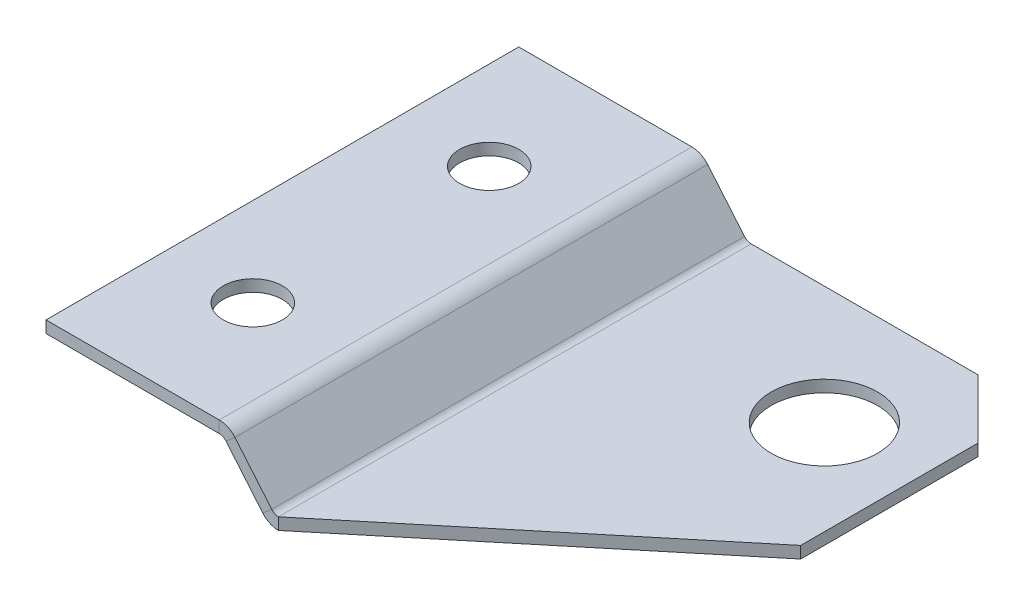
ISO-10303-21;
HEADER;
FILE_DESCRIPTION(('STEP AP214'),'2;1');
FILE_NAME('part.step','',(''),(''),'','','');
FILE_SCHEMA(('AUTOMOTIVE_DESIGN { 1 0 10303 214 1 1 1 1 }'));
ENDSEC;
DATA;
#1=APPLICATION_CONTEXT('core data for automotive mechanical design processes');
#2=APPLICATION_PROTOCOL_DEFINITION('international standard','automotive_design',2000,#1);
#3=PRODUCT_CONTEXT('',#1,'mechanical');
#4=PRODUCT('Part','Part','',(#3));
#5=PRODUCT_RELATED_PRODUCT_CATEGORY('part','',(#4));
#6=PRODUCT_DEFINITION_FORMATION('','',#4);
#7=PRODUCT_DEFINITION_CONTEXT('part definition',#1,'design');
#8=PRODUCT_DEFINITION('design','',#6,#7);
#9=PRODUCT_DEFINITION_SHAPE('','',#8);
#10=(LENGTH_UNIT() NAMED_UNIT(*) SI_UNIT(.MILLI.,.METRE.));
#11=(NAMED_UNIT(*) PLANE_ANGLE_UNIT() SI_UNIT($,.RADIAN.));
#12=(NAMED_UNIT(*) SI_UNIT($,.STERADIAN.) SOLID_ANGLE_UNIT());
#13=UNCERTAINTY_MEASURE_WITH_UNIT(LENGTH_MEASURE(1.E-05),#10,'distance_accuracy_value','');
#14=(GEOMETRIC_REPRESENTATION_CONTEXT(3) GLOBAL_UNCERTAINTY_ASSIGNED_CONTEXT((#13)) GLOBAL_UNIT_ASSIGNED_CONTEXT((#10,
#11,#12)) REPRESENTATION_CONTEXT('',''));
#15=CARTESIAN_POINT('',(0.,0.,0.));
#16=DIRECTION('',(0.,0.,1.));
#17=DIRECTION('',(1.,0.,0.));
#18=AXIS2_PLACEMENT_3D('',#15,#16,#17);
#19=CARTESIAN_POINT('',(19.3230333162743,-4.59626665871385,-40.));
#20=DIRECTION('',(0.,0.,-1.));
#21=DIRECTION('',(-1.,0.,0.));
#22=AXIS2_PLACEMENT_3D('',#19,#20,#21);
#23=PLANE('',#22);
#24=DIRECTION('',(0.642787609686543,-0.766044443118975,0.));
#25=VECTOR('',#24,1.);
#26=CARTESIAN_POINT('',(19.3230333162743,-4.59626665871385,-40.));
#27=LINE('',#26,#25);
#28=CARTESIAN_POINT('',(15.9868305589234,-0.620335037018352,-40.));
#29=VERTEX_POINT('',#28);
#30=CARTESIAN_POINT('',(19.1022472004698,-4.33314401200895,-40.));
#31=VERTEX_POINT('',#30);
#32=EDGE_CURVE('E211',#29,#31,#27,.T.);
#33=ORIENTED_EDGE('',*,*,#32,.T.);
#34=DIRECTION('',(-0.766044443118976,-0.642787609686542,0.));
#35=VECTOR('',#34,1.);
#36=CARTESIAN_POINT('',(19.1022472004698,-4.33314401200896,-40.));
#37=LINE('',#36,#35);
#38=CARTESIAN_POINT('',(18.3362027573508,-4.9759316216955,-40.));
#39=VERTEX_POINT('',#38);
#40=EDGE_CURVE('E194',#31,#39,#37,.T.);
#41=ORIENTED_EDGE('',*,*,#40,.T.);
#42=DIRECTION('',(0.642787609686543,-0.766044443118975,0.));
#43=VECTOR('',#42,1.);
#44=CARTESIAN_POINT('',(18.5569888731553,-5.23905426840039,-40.));
#45=LINE('',#44,#43);
#46=CARTESIAN_POINT('',(15.2207861158045,-1.26312264670489,-40.));
#47=VERTEX_POINT('',#46);
#48=EDGE_CURVE('E214',#47,#39,#45,.T.);
#49=ORIENTED_EDGE('',*,*,#48,.F.);
#50=DIRECTION('',(0.766044443118975,0.642787609686543,0.));
#51=VECTOR('',#50,1.);
#52=CARTESIAN_POINT('',(15.2207861158045,-1.26312264670489,-40.));
#53=LINE('',#52,#51);
#54=EDGE_CURVE('E196',#47,#29,#53,.T.);
#55=ORIENTED_EDGE('',*,*,#54,.T.);
#56=EDGE_LOOP('',(#33,#41,#49,#55));
#57=FACE_BOUND('',#56,.T.);
#58=ADVANCED_FACE('F43',(#57),#23,.T.);
#59=CARTESIAN_POINT('',(9.07600189911477,7.61566984611158,0.));
#60=DIRECTION('',(0.766044443118975,0.642787609686543,0.));
#61=DIRECTION('',(-0.642787609686543,0.766044443118975,0.));
#62=AXIS2_PLACEMENT_3D('',#59,#60,#61);
#63=PLANE('',#62);
#64=DIRECTION('',(-0.642787609686543,0.766044443118975,0.));
#65=VECTOR('',#64,1.);
#66=CARTESIAN_POINT('',(15.766044443119,-0.357212390313457,0.));
#67=LINE('',#66,#65);
#68=CARTESIAN_POINT('',(19.1022472004698,-4.33314401200896,0.));
#69=VERTEX_POINT('',#68);
#70=CARTESIAN_POINT('',(15.9868305589234,-0.620335037018351,0.));
#71=VERTEX_POINT('',#70);
#72=EDGE_CURVE('E216',#69,#71,#67,.T.);
#73=ORIENTED_EDGE('',*,*,#72,.F.);
#74=DIRECTION('',(0.,0.,-1.));
#75=VECTOR('',#74,1.);
#76=CARTESIAN_POINT('',(19.1022472004698,-4.33314401200896,-40.));
#77=LINE('',#76,#75);
#78=EDGE_CURVE('E161',#31,#69,#77,.F.);
#79=ORIENTED_EDGE('',*,*,#78,.F.);
#80=ORIENTED_EDGE('',*,*,#32,.F.);
#81=DIRECTION('',(0.,0.,1.));
#82=VECTOR('',#81,1.);
#83=CARTESIAN_POINT('',(15.9868305589234,-0.620335037018349,0.));
#84=LINE('',#83,#82);
#85=EDGE_CURVE('E206',#29,#71,#84,.T.);
#86=ORIENTED_EDGE('',*,*,#85,.T.);
#87=EDGE_LOOP('',(#73,#79,#80,#86));
#88=FACE_BOUND('',#87,.T.);
#89=ADVANCED_FACE('F301',(#88),#63,.T.);
#90=CARTESIAN_POINT('',(8.3099574559958,6.97288223642504,0.));
#91=DIRECTION('',(0.766044443118975,0.642787609686543,0.));
#92=DIRECTION('',(-0.642787609686543,0.766044443118975,0.));
#93=AXIS2_PLACEMENT_3D('',#90,#91,#92);
#94=PLANE('',#93);
#95=DIRECTION('',(0.,0.,-1.));
#96=VECTOR('',#95,1.);
#97=CARTESIAN_POINT('',(18.3362027573508,-4.9759316216955,-40.));
#98=LINE('',#97,#96);
#99=CARTESIAN_POINT('',(18.3362027573508,-4.9759316216955,0.));
#100=VERTEX_POINT('',#99);
#101=EDGE_CURVE('E188',#39,#100,#98,.F.);
#102=ORIENTED_EDGE('',*,*,#101,.T.);
#103=DIRECTION('',(-0.642787609686543,0.766044443118975,0.));
#104=VECTOR('',#103,1.);
#105=CARTESIAN_POINT('',(15.,-1.,0.));
#106=LINE('',#105,#104);
#107=CARTESIAN_POINT('',(15.2207861158045,-1.26312264670489,0.));
#108=VERTEX_POINT('',#107);
#109=EDGE_CURVE('E220',#100,#108,#106,.T.);
#110=ORIENTED_EDGE('',*,*,#109,.T.);
#111=DIRECTION('',(0.,0.,1.));
#112=VECTOR('',#111,1.);
#113=CARTESIAN_POINT('',(15.2207861158045,-1.26312264670489,-40.));
#114=LINE('',#113,#112);
#115=EDGE_CURVE('E201',#47,#108,#114,.T.);
#116=ORIENTED_EDGE('',*,*,#115,.F.);
#117=ORIENTED_EDGE('',*,*,#48,.T.);
#118=EDGE_LOOP('',(#102,#110,#116,#117));
#119=FACE_BOUND('',#118,.T.);
#120=ADVANCED_FACE('F290',(#119),#94,.F.);
#121=CARTESIAN_POINT('',(0.,-1.,0.));
#122=DIRECTION('',(0.,0.,1.));
#123=DIRECTION('',(1.,0.,0.));
#124=AXIS2_PLACEMENT_3D('',#121,#122,#123);
#125=PLANE('',#124);
#126=DIRECTION('',(1.,0.,0.));
#127=VECTOR('',#126,1.);
#128=CARTESIAN_POINT('',(0.,-1.,0.));
#129=LINE('',#128,#127);
#130=CARTESIAN_POINT('',(0.,-1.,0.));
#131=VERTEX_POINT('',#130);
#132=CARTESIAN_POINT('',(14.656517779003,-1.,0.));
#133=VERTEX_POINT('',#132);
#134=EDGE_CURVE('E248',#131,#133,#129,.T.);
#135=ORIENTED_EDGE('',*,*,#134,.T.);
#136=DIRECTION('',(0.,1.,0.));
#137=VECTOR('',#136,1.);
#138=CARTESIAN_POINT('',(14.656517779003,-1.,0.));
#139=LINE('',#138,#137);
#140=CARTESIAN_POINT('',(14.656517779003,0.,0.));
#141=VERTEX_POINT('',#140);
#142=EDGE_CURVE('E229',#133,#141,#139,.T.);
#143=ORIENTED_EDGE('',*,*,#142,.T.);
#144=DIRECTION('',(1.,0.,0.));
#145=VECTOR('',#144,1.);
#146=CARTESIAN_POINT('',(0.,0.,0.));
#147=LINE('',#146,#145);
#148=CARTESIAN_POINT('',(0.,0.,0.));
#149=VERTEX_POINT('',#148);
#150=EDGE_CURVE('E259',#149,#141,#147,.T.);
#151=ORIENTED_EDGE('',*,*,#150,.F.);
#152=DIRECTION('',(0.,1.,0.));
#153=VECTOR('',#152,1.);
#154=CARTESIAN_POINT('',(0.,-1.,0.));
#155=LINE('',#154,#153);
#156=EDGE_CURVE('E253',#131,#149,#155,.T.);
#157=ORIENTED_EDGE('',*,*,#156,.F.);
#158=EDGE_LOOP('',(#135,#143,#151,#157));
#159=FACE_BOUND('',#158,.T.);
#160=ADVANCED_FACE('F333',(#159),#125,.T.);
#161=CARTESIAN_POINT('',(0.,-1.,0.));
#162=DIRECTION('',(0.,-1.,0.));
#163=DIRECTION('',(0.,0.,-1.));
#164=AXIS2_PLACEMENT_3D('',#161,#162,#163);
#165=PLANE('',#164);
#166=CARTESIAN_POINT('',(7.5,-0.999999999999999,-10.));
#167=DIRECTION('',(0.,-1.,0.));
#168=DIRECTION('',(0.,0.,-1.));
#169=AXIS2_PLACEMENT_3D('',#166,#167,#168);
#170=CIRCLE('',#169,2.5);
#171=CARTESIAN_POINT('',(7.5,-0.999999999999999,-12.5));
#172=VERTEX_POINT('',#171);
#173=EDGE_CURVE('E158',#172,#172,#170,.T.);
#174=ORIENTED_EDGE('',*,*,#173,.F.);
#175=EDGE_LOOP('',(#174));
#176=FACE_BOUND('',#175,.T.);
#177=CARTESIAN_POINT('',(7.5,-0.999999999999999,-30.));
#178=DIRECTION('',(0.,-1.,0.));
#179=DIRECTION('',(0.,0.,-1.));
#180=AXIS2_PLACEMENT_3D('',#177,#178,#179);
#181=CIRCLE('',#180,2.5);
#182=CARTESIAN_POINT('',(7.5,-0.999999999999999,-32.5));
#183=VERTEX_POINT('',#182);
#184=EDGE_CURVE('E611',#183,#183,#181,.T.);
#185=ORIENTED_EDGE('',*,*,#184,.F.);
#186=EDGE_LOOP('',(#185));
#187=FACE_BOUND('',#186,.T.);
#188=DIRECTION('',(-1.,0.,0.));
#189=VECTOR('',#188,1.);
#190=CARTESIAN_POINT('',(0.,-1.,-40.));
#191=LINE('',#190,#189);
#192=CARTESIAN_POINT('',(14.656517779003,-1.,-40.));
#193=VERTEX_POINT('',#192);
#194=CARTESIAN_POINT('',(0.,-1.,-40.));
#195=VERTEX_POINT('',#194);
#196=EDGE_CURVE('E254',#193,#195,#191,.T.);
#197=ORIENTED_EDGE('',*,*,#196,.F.);
#198=DIRECTION('',(0.,0.,1.));
#199=VECTOR('',#198,1.);
#200=CARTESIAN_POINT('',(14.656517779003,-1.,0.));
#201=LINE('',#200,#199);
#202=EDGE_CURVE('E236',#133,#193,#201,.F.);
#203=ORIENTED_EDGE('',*,*,#202,.F.);
#204=ORIENTED_EDGE('',*,*,#134,.F.);
#205=DIRECTION('',(0.,0.,1.));
#206=VECTOR('',#205,1.);
#207=CARTESIAN_POINT('',(0.,-1.,0.));
#208=LINE('',#207,#206);
#209=EDGE_CURVE('E246',#195,#131,#208,.T.);
#210=ORIENTED_EDGE('',*,*,#209,.F.);
#211=EDGE_LOOP('',(#197,#203,#204,#210));
#212=FACE_BOUND('',#211,.T.);
#213=ADVANCED_FACE('F326',(#176,#187,#212),#165,.T.);
#214=CARTESIAN_POINT('',(0.,0.,0.));
#215=DIRECTION('',(0.,-1.,0.));
#216=DIRECTION('',(0.,0.,-1.));
#217=AXIS2_PLACEMENT_3D('',#214,#215,#216);
#218=PLANE('',#217);
#219=CARTESIAN_POINT('',(7.5,0.,-10.));
#220=DIRECTION('',(0.,1.,0.));
#221=DIRECTION('',(0.,0.,1.));
#222=AXIS2_PLACEMENT_3D('',#219,#220,#221);
#223=CIRCLE('',#222,2.5);
#224=CARTESIAN_POINT('',(7.5,0.,-7.5));
#225=VERTEX_POINT('',#224);
#226=EDGE_CURVE('E607',#225,#225,#223,.T.);
#227=ORIENTED_EDGE('',*,*,#226,.F.);
#228=EDGE_LOOP('',(#227));
#229=FACE_BOUND('',#228,.T.);
#230=CARTESIAN_POINT('',(7.5,0.,-30.));
#231=DIRECTION('',(0.,1.,0.));
#232=DIRECTION('',(0.,0.,1.));
#233=AXIS2_PLACEMENT_3D('',#230,#231,#232);
#234=CIRCLE('',#233,2.5);
#235=CARTESIAN_POINT('',(7.5,0.,-27.5));
#236=VERTEX_POINT('',#235);
#237=EDGE_CURVE('E608',#236,#236,#234,.T.);
#238=ORIENTED_EDGE('',*,*,#237,.F.);
#239=EDGE_LOOP('',(#238));
#240=FACE_BOUND('',#239,.T.);
#241=DIRECTION('',(0.,0.,1.));
#242=VECTOR('',#241,1.);
#243=CARTESIAN_POINT('',(14.656517779003,0.,0.));
#244=LINE('',#243,#242);
#245=CARTESIAN_POINT('',(14.656517779003,0.,-40.));
#246=VERTEX_POINT('',#245);
#247=EDGE_CURVE('E224',#141,#246,#244,.F.);
#248=ORIENTED_EDGE('',*,*,#247,.T.);
#249=DIRECTION('',(-1.,0.,0.));
#250=VECTOR('',#249,1.);
#251=CARTESIAN_POINT('',(0.,0.,-40.));
#252=LINE('',#251,#250);
#253=CARTESIAN_POINT('',(0.,0.,-40.));
#254=VERTEX_POINT('',#253);
#255=EDGE_CURVE('E249',#246,#254,#252,.T.);
#256=ORIENTED_EDGE('',*,*,#255,.T.);
#257=DIRECTION('',(0.,0.,1.));
#258=VECTOR('',#257,1.);
#259=CARTESIAN_POINT('',(0.,0.,0.));
#260=LINE('',#259,#258);
#261=EDGE_CURVE('E242',#254,#149,#260,.T.);
#262=ORIENTED_EDGE('',*,*,#261,.T.);
#263=ORIENTED_EDGE('',*,*,#150,.T.);
#264=EDGE_LOOP('',(#248,#256,#262,#263));
#265=FACE_BOUND('',#264,.T.);
#266=ADVANCED_FACE('F335',(#229,#240,#265),#218,.F.);
#267=CARTESIAN_POINT('',(0.,-1.,0.));
#268=DIRECTION('',(-1.,0.,0.));
#269=DIRECTION('',(0.,0.,1.));
#270=AXIS2_PLACEMENT_3D('',#267,#268,#269);
#271=PLANE('',#270);
#272=ORIENTED_EDGE('',*,*,#261,.F.);
#273=DIRECTION('',(0.,1.,0.));
#274=VECTOR('',#273,1.);
#275=CARTESIAN_POINT('',(0.,-1.,-40.));
#276=LINE('',#275,#274);
#277=EDGE_CURVE('E264',#195,#254,#276,.T.);
#278=ORIENTED_EDGE('',*,*,#277,.F.);
#279=ORIENTED_EDGE('',*,*,#209,.T.);
#280=ORIENTED_EDGE('',*,*,#156,.T.);
#281=EDGE_LOOP('',(#272,#278,#279,#280));
#282=FACE_BOUND('',#281,.T.);
#283=ADVANCED_FACE('F44',(#282),#271,.T.);
#284=CARTESIAN_POINT('',(0.,-1.,-40.));
#285=DIRECTION('',(0.,0.,-1.));
#286=DIRECTION('',(-1.,0.,0.));
#287=AXIS2_PLACEMENT_3D('',#284,#285,#286);
#288=PLANE('',#287);
#289=DIRECTION('',(0.,1.,0.));
#290=VECTOR('',#289,1.);
#291=CARTESIAN_POINT('',(14.656517779003,-1.,-40.));
#292=LINE('',#291,#290);
#293=EDGE_CURVE('E241',#193,#246,#292,.T.);
#294=ORIENTED_EDGE('',*,*,#293,.F.);
#295=ORIENTED_EDGE('',*,*,#196,.T.);
#296=ORIENTED_EDGE('',*,*,#277,.T.);
#297=ORIENTED_EDGE('',*,*,#255,.F.);
#298=EDGE_LOOP('',(#294,#295,#296,#297));
#299=FACE_BOUND('',#298,.T.);
#300=ADVANCED_FACE('F329',(#299),#288,.T.);
#301=CARTESIAN_POINT('',(14.656517779003,-1.7366,-40.));
#302=DIRECTION('',(0.,0.,-1.));
#303=DIRECTION('',(-1.,0.,0.));
#304=AXIS2_PLACEMENT_3D('',#301,#302,#303);
#305=PLANE('',#304);
#306=ORIENTED_EDGE('',*,*,#54,.F.);
#307=CARTESIAN_POINT('',(14.656517779003,-1.7366,-40.));
#308=DIRECTION('',(0.,0.,1.));
#309=DIRECTION('',(1.,0.,0.));
#310=AXIS2_PLACEMENT_3D('',#307,#308,#309);
#311=CIRCLE('',#310,0.736600000000002);
#312=EDGE_CURVE('E231',#193,#47,#311,.F.);
#313=ORIENTED_EDGE('',*,*,#312,.F.);
#314=ORIENTED_EDGE('',*,*,#293,.T.);
#315=CARTESIAN_POINT('',(14.656517779003,-1.7366,-40.));
#316=DIRECTION('',(0.,0.,1.));
#317=DIRECTION('',(1.,0.,0.));
#318=AXIS2_PLACEMENT_3D('',#315,#316,#317);
#319=CIRCLE('',#318,1.7366);
#320=EDGE_CURVE('E228',#246,#29,#319,.F.);
#321=ORIENTED_EDGE('',*,*,#320,.T.);
#322=EDGE_LOOP('',(#306,#313,#314,#321));
#323=FACE_BOUND('',#322,.T.);
#324=ADVANCED_FACE('F310',(#323),#305,.T.);
#325=CARTESIAN_POINT('',(14.656517779003,-1.7366,0.));
#326=DIRECTION('',(0.,0.,-1.));
#327=DIRECTION('',(-1.,0.,0.));
#328=AXIS2_PLACEMENT_3D('',#325,#326,#327);
#329=PLANE('',#328);
#330=CARTESIAN_POINT('',(14.656517779003,-1.7366,0.));
#331=DIRECTION('',(0.,0.,1.));
#332=DIRECTION('',(1.,0.,0.));
#333=AXIS2_PLACEMENT_3D('',#330,#331,#332);
#334=CIRCLE('',#333,0.736600000000002);
#335=EDGE_CURVE('E217',#108,#133,#334,.T.);
#336=ORIENTED_EDGE('',*,*,#335,.F.);
#337=DIRECTION('',(0.766044443118975,0.642787609686543,0.));
#338=VECTOR('',#337,1.);
#339=CARTESIAN_POINT('',(15.2207861158045,-1.26312264670489,0.));
#340=LINE('',#339,#338);
#341=EDGE_CURVE('E202',#108,#71,#340,.T.);
#342=ORIENTED_EDGE('',*,*,#341,.T.);
#343=CARTESIAN_POINT('',(14.656517779003,-1.7366,0.));
#344=DIRECTION('',(0.,0.,1.));
#345=DIRECTION('',(1.,0.,0.));
#346=AXIS2_PLACEMENT_3D('',#343,#344,#345);
#347=CIRCLE('',#346,1.7366);
#348=EDGE_CURVE('E227',#71,#141,#347,.T.);
#349=ORIENTED_EDGE('',*,*,#348,.T.);
#350=ORIENTED_EDGE('',*,*,#142,.F.);
#351=EDGE_LOOP('',(#336,#342,#349,#350));
#352=FACE_BOUND('',#351,.T.);
#353=ADVANCED_FACE('F300',(#352),#329,.F.);
#354=CARTESIAN_POINT('',(14.656517779003,-1.7366,0.));
#355=DIRECTION('',(0.,0.,1.));
#356=DIRECTION('',(0.766044443118975,0.642787609686543,0.));
#357=AXIS2_PLACEMENT_3D('',#354,#355,#356);
#358=CYLINDRICAL_SURFACE('',#357,1.7366);
#359=ORIENTED_EDGE('',*,*,#247,.F.);
#360=ORIENTED_EDGE('',*,*,#348,.F.);
#361=ORIENTED_EDGE('',*,*,#85,.F.);
#362=ORIENTED_EDGE('',*,*,#320,.F.);
#363=EDGE_LOOP('',(#359,#360,#361,#362));
#364=FACE_BOUND('',#363,.T.);
#365=ADVANCED_FACE('F304',(#364),#358,.T.);
#366=CARTESIAN_POINT('',(14.656517779003,-1.7366,0.));
#367=DIRECTION('',(0.,0.,1.));
#368=DIRECTION('',(0.766044443118975,0.642787609686543,0.));
#369=AXIS2_PLACEMENT_3D('',#366,#367,#368);
#370=CYLINDRICAL_SURFACE('',#369,0.736600000000002);
#371=ORIENTED_EDGE('',*,*,#202,.T.);
#372=ORIENTED_EDGE('',*,*,#312,.T.);
#373=ORIENTED_EDGE('',*,*,#115,.T.);
#374=ORIENTED_EDGE('',*,*,#335,.T.);
#375=EDGE_LOOP('',(#371,#372,#373,#374));
#376=FACE_BOUND('',#375,.T.);
#377=ADVANCED_FACE('F325',(#376),#370,.F.);
#378=CARTESIAN_POINT('',(15.766044443119,-0.357212390313457,0.));
#379=DIRECTION('',(0.,0.,1.));
#380=DIRECTION('',(1.,0.,0.));
#381=AXIS2_PLACEMENT_3D('',#378,#379,#380);
#382=PLANE('',#381);
#383=DIRECTION('',(-0.766044443118976,-0.642787609686542,0.));
#384=VECTOR('',#383,1.);
#385=CARTESIAN_POINT('',(19.1022472004698,-4.33314401200896,0.));
#386=LINE('',#385,#384);
#387=EDGE_CURVE('E197',#69,#100,#386,.T.);
#388=ORIENTED_EDGE('',*,*,#387,.F.);
#389=ORIENTED_EDGE('',*,*,#72,.T.);
#390=ORIENTED_EDGE('',*,*,#341,.F.);
#391=ORIENTED_EDGE('',*,*,#109,.F.);
#392=EDGE_LOOP('',(#388,#389,#390,#391));
#393=FACE_BOUND('',#392,.T.);
#394=ADVANCED_FACE('F292',(#393),#382,.T.);
#395=CARTESIAN_POINT('',(19.6665155372712,-3.85966665871385,0.));
#396=DIRECTION('',(0.,0.,1.));
#397=DIRECTION('',(1.,0.,0.));
#398=AXIS2_PLACEMENT_3D('',#395,#396,#397);
#399=PLANE('',#398);
#400=DIRECTION('',(0.,-1.,0.));
#401=VECTOR('',#400,1.);
#402=CARTESIAN_POINT('',(19.6665155372712,-4.59626665871385,0.));
#403=LINE('',#402,#401);
#404=CARTESIAN_POINT('',(19.6665155372712,-4.59626665871385,0.));
#405=VERTEX_POINT('',#404);
#406=CARTESIAN_POINT('',(19.6665155372712,-5.59626665871385,0.));
#407=VERTEX_POINT('',#406);
#408=EDGE_CURVE('E140',#405,#407,#403,.T.);
#409=ORIENTED_EDGE('',*,*,#408,.F.);
#410=CARTESIAN_POINT('',(19.6665155372712,-3.85966665871385,0.));
#411=DIRECTION('',(0.,0.,-1.));
#412=DIRECTION('',(-1.,0.,0.));
#413=AXIS2_PLACEMENT_3D('',#410,#411,#412);
#414=CIRCLE('',#413,0.736599999999999);
#415=EDGE_CURVE('E151',#69,#405,#414,.F.);
#416=ORIENTED_EDGE('',*,*,#415,.F.);
#417=ORIENTED_EDGE('',*,*,#387,.T.);
#418=CARTESIAN_POINT('',(19.6665155372712,-3.85966665871385,0.));
#419=DIRECTION('',(0.,0.,-1.));
#420=DIRECTION('',(-1.,0.,0.));
#421=AXIS2_PLACEMENT_3D('',#418,#419,#420);
#422=CIRCLE('',#421,1.7366);
#423=EDGE_CURVE('E153',#100,#407,#422,.F.);
#424=ORIENTED_EDGE('',*,*,#423,.T.);
#425=EDGE_LOOP('',(#409,#416,#417,#424));
#426=FACE_BOUND('',#425,.T.);
#427=ADVANCED_FACE('F148',(#426),#399,.T.);
#428=CARTESIAN_POINT('',(19.6665155372712,-3.85966665871385,-40.));
#429=DIRECTION('',(0.,0.,1.));
#430=DIRECTION('',(1.,0.,0.));
#431=AXIS2_PLACEMENT_3D('',#428,#429,#430);
#432=PLANE('',#431);
#433=CARTESIAN_POINT('',(19.6665155372712,-3.85966665871385,-40.));
#434=DIRECTION('',(0.,0.,-1.));
#435=DIRECTION('',(-1.,0.,0.));
#436=AXIS2_PLACEMENT_3D('',#433,#434,#435);
#437=CIRCLE('',#436,0.736599999999999);
#438=CARTESIAN_POINT('',(19.6665155372712,-4.59626665871385,-40.));
#439=VERTEX_POINT('',#438);
#440=EDGE_CURVE('E190',#439,#31,#437,.T.);
#441=ORIENTED_EDGE('',*,*,#440,.F.);
#442=DIRECTION('',(0.,-1.,0.));
#443=VECTOR('',#442,1.);
#444=CARTESIAN_POINT('',(19.6665155372712,-4.59626665871385,-40.));
#445=LINE('',#444,#443);
#446=CARTESIAN_POINT('',(19.6665155372712,-5.59626665871385,-40.));
#447=VERTEX_POINT('',#446);
#448=EDGE_CURVE('E167',#439,#447,#445,.T.);
#449=ORIENTED_EDGE('',*,*,#448,.T.);
#450=CARTESIAN_POINT('',(19.6665155372712,-3.85966665871385,-40.));
#451=DIRECTION('',(0.,0.,-1.));
#452=DIRECTION('',(-1.,0.,0.));
#453=AXIS2_PLACEMENT_3D('',#450,#451,#452);
#454=CIRCLE('',#453,1.7366);
#455=EDGE_CURVE('E165',#447,#39,#454,.T.);
#456=ORIENTED_EDGE('',*,*,#455,.T.);
#457=ORIENTED_EDGE('',*,*,#40,.F.);
#458=EDGE_LOOP('',(#441,#449,#456,#457));
#459=FACE_BOUND('',#458,.T.);
#460=ADVANCED_FACE('F279',(#459),#432,.F.);
#461=CARTESIAN_POINT('',(19.6665155372712,-3.85966665871385,-40.));
#462=DIRECTION('',(0.,0.,-1.));
#463=DIRECTION('',(0.,-1.,0.));
#464=AXIS2_PLACEMENT_3D('',#461,#462,#463);
#465=CYLINDRICAL_SURFACE('',#464,1.7366);
#466=ORIENTED_EDGE('',*,*,#101,.F.);
#467=ORIENTED_EDGE('',*,*,#455,.F.);
#468=DIRECTION('',(0.,0.,1.));
#469=VECTOR('',#468,1.);
#470=CARTESIAN_POINT('',(19.6665155372712,-5.59626665871385,0.));
#471=LINE('',#470,#469);
#472=EDGE_CURVE('E173',#447,#407,#471,.T.);
#473=ORIENTED_EDGE('',*,*,#472,.T.);
#474=ORIENTED_EDGE('',*,*,#423,.F.);
#475=EDGE_LOOP('',(#466,#467,#473,#474));
#476=FACE_BOUND('',#475,.T.);
#477=ADVANCED_FACE('F283',(#476),#465,.T.);
#478=CARTESIAN_POINT('',(19.6665155372712,-3.85966665871385,-40.));
#479=DIRECTION('',(0.,0.,-1.));
#480=DIRECTION('',(0.,-1.,0.));
#481=AXIS2_PLACEMENT_3D('',#478,#479,#480);
#482=CYLINDRICAL_SURFACE('',#481,0.736599999999999);
#483=ORIENTED_EDGE('',*,*,#78,.T.);
#484=ORIENTED_EDGE('',*,*,#415,.T.);
#485=DIRECTION('',(0.,0.,-1.));
#486=VECTOR('',#485,1.);
#487=CARTESIAN_POINT('',(19.6665155372712,-4.59626665871385,0.));
#488=LINE('',#487,#486);
#489=EDGE_CURVE('E152',#405,#439,#488,.T.);
#490=ORIENTED_EDGE('',*,*,#489,.T.);
#491=ORIENTED_EDGE('',*,*,#440,.T.);
#492=EDGE_LOOP('',(#483,#484,#490,#491));
#493=FACE_BOUND('',#492,.T.);
#494=ADVANCED_FACE('F157',(#493),#482,.F.);
#495=CARTESIAN_POINT('',(43.8567256581193,-5.59626665871385,-40.));
#496=DIRECTION('',(0.,0.,1.));
#497=DIRECTION('',(1.,0.,0.));
#498=AXIS2_PLACEMENT_3D('',#495,#496,#497);
#499=PLANE('',#498);
#500=DIRECTION('',(1.,0.,0.));
#501=VECTOR('',#500,1.);
#502=CARTESIAN_POINT('',(43.8567256581193,-4.59626665871385,-40.));
#503=LINE('',#502,#501);
#504=CARTESIAN_POINT('',(38.8567256581193,-4.59626665871385,-40.));
#505=VERTEX_POINT('',#504);
#506=EDGE_CURVE('E169',#439,#505,#503,.T.);
#507=ORIENTED_EDGE('',*,*,#506,.T.);
#508=DIRECTION('',(0.,1.,0.));
#509=VECTOR('',#508,1.);
#510=CARTESIAN_POINT('',(38.8567256581193,-14.5962666587139,-40.));
#511=LINE('',#510,#509);
#512=CARTESIAN_POINT('',(38.8567256581193,-5.59626665871385,-40.));
#513=VERTEX_POINT('',#512);
#514=EDGE_CURVE('E144',#513,#505,#511,.T.);
#515=ORIENTED_EDGE('',*,*,#514,.F.);
#516=DIRECTION('',(1.,0.,0.));
#517=VECTOR('',#516,1.);
#518=CARTESIAN_POINT('',(43.8567256581193,-5.59626665871385,-40.));
#519=LINE('',#518,#517);
#520=EDGE_CURVE('E179',#447,#513,#519,.T.);
#521=ORIENTED_EDGE('',*,*,#520,.F.);
#522=ORIENTED_EDGE('',*,*,#448,.F.);
#523=EDGE_LOOP('',(#507,#515,#521,#522));
#524=FACE_BOUND('',#523,.T.);
#525=ADVANCED_FACE('F274',(#524),#499,.F.);
#526=CARTESIAN_POINT('',(0.,-5.59626665871384,0.));
#527=DIRECTION('',(0.,1.,0.));
#528=DIRECTION('',(-1.,0.,0.));
#529=AXIS2_PLACEMENT_3D('',#526,#527,#528);
#530=PLANE('',#529);
#531=CARTESIAN_POINT('',(35.8567256581193,-5.59626665871385,-30.));
#532=DIRECTION('',(0.,1.,0.));
#533=DIRECTION('',(-1.,0.,0.));
#534=AXIS2_PLACEMENT_3D('',#531,#532,#533);
#535=CIRCLE('',#534,4.5);
#536=CARTESIAN_POINT('',(31.3567256581193,-5.59626665871385,-30.));
#537=VERTEX_POINT('',#536);
#538=EDGE_CURVE('E268',#537,#537,#535,.T.);
#539=ORIENTED_EDGE('',*,*,#538,.T.);
#540=EDGE_LOOP('',(#539));
#541=FACE_BOUND('',#540,.T.);
#542=DIRECTION('',(0.,0.,1.));
#543=VECTOR('',#542,1.);
#544=CARTESIAN_POINT('',(43.8567256581193,-5.59626665871385,0.));
#545=LINE('',#544,#543);
#546=CARTESIAN_POINT('',(43.8567256581193,-5.59626665871385,-35.));
#547=VERTEX_POINT('',#546);
#548=CARTESIAN_POINT('',(43.8567256581193,-5.59626665871385,-20.));
#549=VERTEX_POINT('',#548);
#550=EDGE_CURVE('E182',#547,#549,#545,.T.);
#551=ORIENTED_EDGE('',*,*,#550,.T.);
#552=DIRECTION('',(-0.770699140484971,0.,0.6371992112799));
#553=VECTOR('',#552,1.);
#554=CARTESIAN_POINT('',(7.98505439017706,-5.59626665871385,9.65800717623915));
#555=LINE('',#554,#553);
#556=EDGE_CURVE('E59',#549,#407,#555,.T.);
#557=ORIENTED_EDGE('',*,*,#556,.T.);
#558=ORIENTED_EDGE('',*,*,#472,.F.);
#559=ORIENTED_EDGE('',*,*,#520,.T.);
#560=DIRECTION('',(0.707106781186548,0.,0.707106781186548));
#561=VECTOR('',#560,1.);
#562=CARTESIAN_POINT('',(39.4283628290596,-5.59626665871385,-39.4283628290596));
#563=LINE('',#562,#561);
#564=EDGE_CURVE('E141',#513,#547,#563,.T.);
#565=ORIENTED_EDGE('',*,*,#564,.T.);
#566=EDGE_LOOP('',(#551,#557,#558,#559,#565));
#567=FACE_BOUND('',#566,.T.);
#568=ADVANCED_FACE('F284',(#541,#567),#530,.F.);
#569=CARTESIAN_POINT('',(0.,-4.59626665871384,0.));
#570=DIRECTION('',(0.,1.,0.));
#571=DIRECTION('',(-1.,0.,0.));
#572=AXIS2_PLACEMENT_3D('',#569,#570,#571);
#573=PLANE('',#572);
#574=CARTESIAN_POINT('',(35.8567256581193,-4.59626665871385,-30.));
#575=DIRECTION('',(0.,1.,0.));
#576=DIRECTION('',(-1.,0.,0.));
#577=AXIS2_PLACEMENT_3D('',#574,#575,#576);
#578=CIRCLE('',#577,4.5);
#579=CARTESIAN_POINT('',(31.3567256581193,-4.59626665871385,-30.));
#580=VERTEX_POINT('',#579);
#581=EDGE_CURVE('E598',#580,#580,#578,.T.);
#582=ORIENTED_EDGE('',*,*,#581,.F.);
#583=EDGE_LOOP('',(#582));
#584=FACE_BOUND('',#583,.T.);
#585=DIRECTION('',(-0.770699140484971,0.,0.6371992112799));
#586=VECTOR('',#585,1.);
#587=CARTESIAN_POINT('',(43.8567256581193,-4.59626665871385,-20.));
#588=LINE('',#587,#586);
#589=CARTESIAN_POINT('',(43.8567256581193,-4.59626665871385,-20.));
#590=VERTEX_POINT('',#589);
#591=EDGE_CURVE('E131',#590,#405,#588,.T.);
#592=ORIENTED_EDGE('',*,*,#591,.F.);
#593=DIRECTION('',(0.,0.,1.));
#594=VECTOR('',#593,1.);
#595=CARTESIAN_POINT('',(43.8567256581193,-4.59626665871385,0.));
#596=LINE('',#595,#594);
#597=CARTESIAN_POINT('',(43.8567256581193,-4.59626665871385,-35.));
#598=VERTEX_POINT('',#597);
#599=EDGE_CURVE('E183',#598,#590,#596,.T.);
#600=ORIENTED_EDGE('',*,*,#599,.F.);
#601=DIRECTION('',(0.707106781186547,0.,0.707106781186547));
#602=VECTOR('',#601,1.);
#603=CARTESIAN_POINT('',(38.8567256581193,-4.59626665871385,-40.));
#604=LINE('',#603,#602);
#605=EDGE_CURVE('E63',#505,#598,#604,.T.);
#606=ORIENTED_EDGE('',*,*,#605,.F.);
#607=ORIENTED_EDGE('',*,*,#506,.F.);
#608=ORIENTED_EDGE('',*,*,#489,.F.);
#609=EDGE_LOOP('',(#592,#600,#606,#607,#608));
#610=FACE_BOUND('',#609,.T.);
#611=ADVANCED_FACE('F170',(#584,#610),#573,.T.);
#612=CARTESIAN_POINT('',(43.8567256581193,-5.59626665871385,0.));
#613=DIRECTION('',(-1.,0.,0.));
#614=DIRECTION('',(0.,-1.,0.));
#615=AXIS2_PLACEMENT_3D('',#612,#613,#614);
#616=PLANE('',#615);
#617=ORIENTED_EDGE('',*,*,#599,.T.);
#618=DIRECTION('',(0.,-1.,0.));
#619=VECTOR('',#618,1.);
#620=CARTESIAN_POINT('',(43.8567256581193,-5.59626665871385,-20.));
#621=LINE('',#620,#619);
#622=EDGE_CURVE('E11',#590,#549,#621,.T.);
#623=ORIENTED_EDGE('',*,*,#622,.T.);
#624=ORIENTED_EDGE('',*,*,#550,.F.);
#625=DIRECTION('',(0.,1.,0.));
#626=VECTOR('',#625,1.);
#627=CARTESIAN_POINT('',(43.8567256581193,-5.59626665871385,-35.));
#628=LINE('',#627,#626);
#629=EDGE_CURVE('E51',#547,#598,#628,.T.);
#630=ORIENTED_EDGE('',*,*,#629,.T.);
#631=EDGE_LOOP('',(#617,#623,#624,#630));
#632=FACE_BOUND('',#631,.T.);
#633=ADVANCED_FACE('F266',(#632),#616,.F.);
#634=CARTESIAN_POINT('',(7.5,-10.,-30.));
#635=DIRECTION('',(0.,1.,0.));
#636=DIRECTION('',(0.,0.,1.));
#637=AXIS2_PLACEMENT_3D('',#634,#635,#636);
#638=CYLINDRICAL_SURFACE('',#637,2.5);
#639=ORIENTED_EDGE('',*,*,#184,.T.);
#640=EDGE_LOOP('',(#639));
#641=FACE_BOUND('',#640,.T.);
#642=ORIENTED_EDGE('',*,*,#237,.T.);
#643=EDGE_LOOP('',(#642));
#644=FACE_BOUND('',#643,.T.);
#645=ADVANCED_FACE('F513',(#641,#644),#638,.F.);
#646=CARTESIAN_POINT('',(7.5,-10.,-10.));
#647=DIRECTION('',(0.,1.,0.));
#648=DIRECTION('',(0.,0.,1.));
#649=AXIS2_PLACEMENT_3D('',#646,#647,#648);
#650=CYLINDRICAL_SURFACE('',#649,2.5);
#651=ORIENTED_EDGE('',*,*,#173,.T.);
#652=EDGE_LOOP('',(#651));
#653=FACE_BOUND('',#652,.T.);
#654=ORIENTED_EDGE('',*,*,#226,.T.);
#655=EDGE_LOOP('',(#654));
#656=FACE_BOUND('',#655,.T.);
#657=ADVANCED_FACE('F529',(#653,#656),#650,.F.);
#658=CARTESIAN_POINT('',(38.8567256581193,-14.5962666587139,-40.));
#659=DIRECTION('',(-0.707106781186548,0.,0.707106781186548));
#660=DIRECTION('',(0.707106781186548,0.,0.707106781186548));
#661=AXIS2_PLACEMENT_3D('',#658,#659,#660);
#662=PLANE('',#661);
#663=ORIENTED_EDGE('',*,*,#514,.T.);
#664=ORIENTED_EDGE('',*,*,#605,.T.);
#665=ORIENTED_EDGE('',*,*,#629,.F.);
#666=ORIENTED_EDGE('',*,*,#564,.F.);
#667=EDGE_LOOP('',(#663,#664,#665,#666));
#668=FACE_BOUND('',#667,.T.);
#669=ADVANCED_FACE('F537',(#668),#662,.F.);
#670=CARTESIAN_POINT('',(43.8567256581193,-14.5962666587139,-20.));
#671=DIRECTION('',(-0.6371992112799,0.,-0.770699140484971));
#672=DIRECTION('',(-0.770699140484971,0.,0.6371992112799));
#673=AXIS2_PLACEMENT_3D('',#670,#671,#672);
#674=PLANE('',#673);
#675=ORIENTED_EDGE('',*,*,#622,.F.);
#676=ORIENTED_EDGE('',*,*,#591,.T.);
#677=ORIENTED_EDGE('',*,*,#408,.T.);
#678=ORIENTED_EDGE('',*,*,#556,.F.);
#679=EDGE_LOOP('',(#675,#676,#677,#678));
#680=FACE_BOUND('',#679,.T.);
#681=ADVANCED_FACE('F136',(#680),#674,.F.);
#682=CARTESIAN_POINT('',(35.8567256581193,-14.5962666587139,-30.));
#683=DIRECTION('',(0.,1.,0.));
#684=DIRECTION('',(-1.,0.,0.));
#685=AXIS2_PLACEMENT_3D('',#682,#683,#684);
#686=CYLINDRICAL_SURFACE('',#685,4.5);
#687=ORIENTED_EDGE('',*,*,#581,.T.);
#688=EDGE_LOOP('',(#687));
#689=FACE_BOUND('',#688,.T.);
#690=ORIENTED_EDGE('',*,*,#538,.F.);
#691=EDGE_LOOP('',(#690));
#692=FACE_BOUND('',#691,.T.);
#693=ADVANCED_FACE('F555',(#689,#692),#686,.F.);
#694=CLOSED_SHELL('',(#58,#89,#120,#160,#213,#266,#283,#300,#324,#353,#365,#377,#394,#427,#460,
#477,#494,#525,#568,#611,#633,#645,#657,#669,#681,#693));
#695=MANIFOLD_SOLID_BREP('B2',#694);
#696=ADVANCED_BREP_SHAPE_REPRESENTATION('',(#18,#695),#14);
#697=SHAPE_DEFINITION_REPRESENTATION(#9,#696);
ENDSEC;
END-ISO-10303-21;
